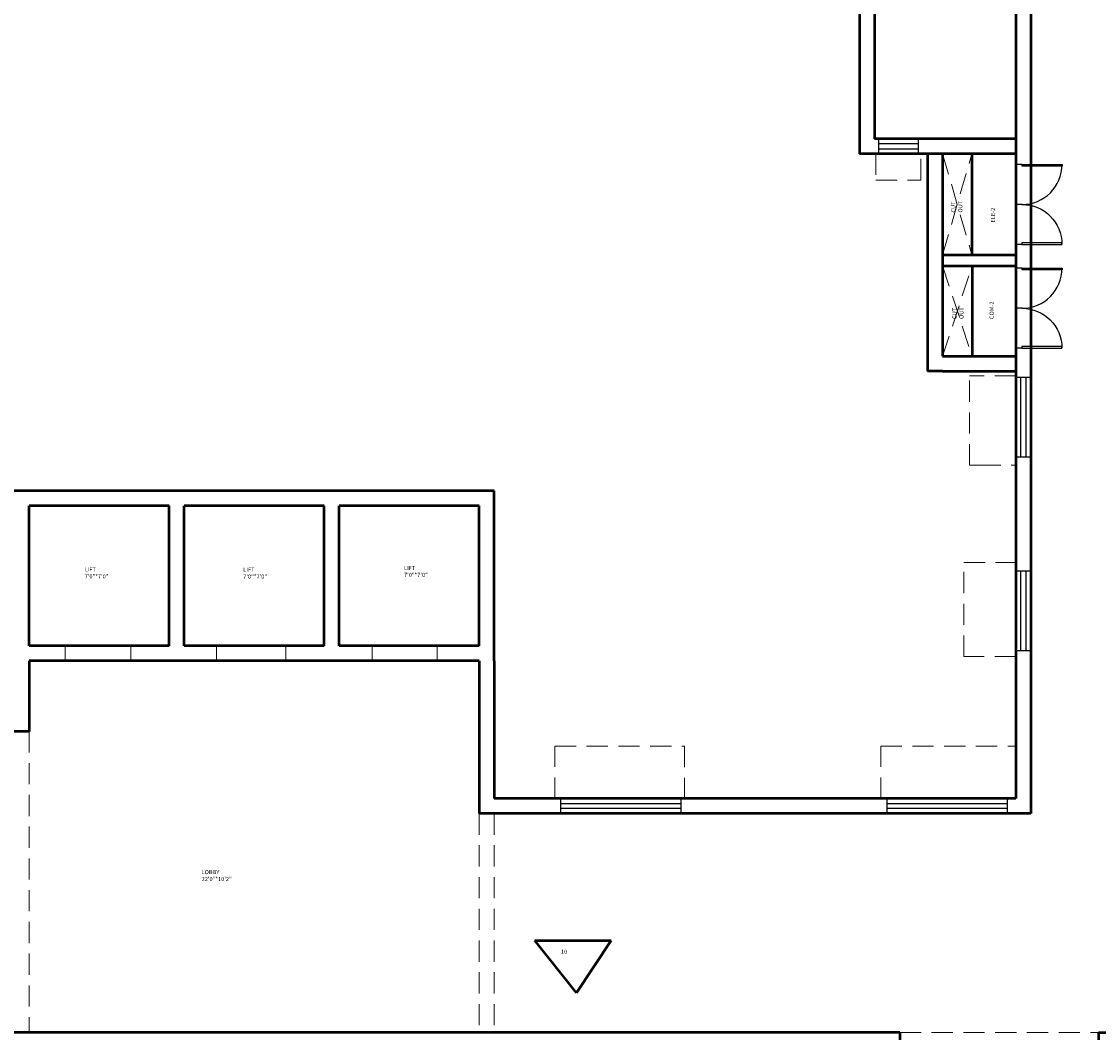
# Model space of a CAD drawing. Units: inches. Extents: x 291 to 2631, y 456 to 2623.
# Tile 9 of 22: x 1463 to 2109, y 931 to 1538. Entities that reach past the tile are written whole.
import ezdxf

# ---------------------------------------------------------------- set-up
doc = ezdxf.new("R2010")
doc.units = ezdxf.units.IN
doc.linetypes.add('DASHED', pattern=[19.05, 12.7, -6.35])
for name, color, linetype, lineweight in [('A-ANNO-TEXT', 3, 'Continuous', 25), ('A-AREA-IDEN', 7, 'Continuous', 25), ('A-DOOR', 3, 'Continuous', 25), ('A-FLOR-OVHD', 1, 'DASHED', 18), ('A-GLAZ', 4, 'Continuous', 25), ('A-WALL', 7, 'Continuous', 50)]:
    doc.layers.add(name, color=color, linetype=linetype, lineweight=lineweight)
doc.styles.get("Standard").update_dxf_attribs({"font": 'arial.ttf'})

# ---------------------------------------------------------------- blocks, each defined once
blk = doc.blocks.new('*U2')
for p, q in [((0, 0), (0, -6)), ((40, 0), (40, -6))]:
    blk.add_line(p, q)
blk.add_lwpolyline([(0, 0), (0, 40), (1.75, 40), (1.75, 0)], close=True)
blk.add_arc((0, 0), 40, 0, 90)
blk = doc.blocks.new('WIN-1800')
for p, q in [((0, 9), (72, 9)), ((0, 0), (0, 9)), ((72, 9), (72, 0)), ((0, 6), (72, 6)), ((72, 3), (0, 3)), ((72, 0), (0, 0))]:
    blk.add_line(p, q)
blk = doc.blocks.new('WIN-1200')
for p, q in [((0, 0), (0, 48)), ((0, 48), (9, 48)), ((3, 0), (3, 48)), ((6, 48), (6, 0)), ((9, 48), (9, 0)), ((9, 0), (0, 0))]:
    blk.add_line(p, q)
blk = doc.blocks.new('WIN-600')
for p, q in [((24, 9), (0, 9)), ((0, 9), (0, 0)), ((24, 0), (24, 9)), ((24, 6), (0, 6)), ((0, 3), (24, 3)), ((0, 0), (24, 0))]:
    blk.add_line(p, q)

msp = doc.modelspace()

# ---------------------------------------------------------------- linework, layer by layer
at = {"layer": 'A-FLOR-OVHD'}
for p, q in [((1975.46, 1458.32), (1975.46, 1442.5)), ((2002.48, 1442.5), (2002.48, 1458.32)), ((2015.46, 1458.32), (2033.04, 1397.55)), ((2015.46, 1397.55), (2033.04, 1458.32)), ((1975.46, 1442.5), (2002.48, 1442.5)), ((2015.46, 1390.95), (2033.18, 1336.78)), ((2015.46, 1336.78), (2033.18, 1390.95)), ((2031.54, 1271.35), (2031.54, 1325.01)), ((2031.54, 1325.01), (2037.66, 1325.01)), ((2059.49, 1325.01), (2037.66, 1325.01)), ((2037.66, 1271.35), (2031.54, 1271.35)), ((2037.66, 1271.35), (2059.49, 1271.35)), ((2028.23, 1156.55), (2028.23, 1213.02)), ((2028.23, 1213.02), (2059.49, 1213.02)), ((1489.28, 1163.05), (1489.28, 1154.05)), ((1528.71, 1163.05), (1528.71, 1154.05)), ((1580.01, 1163.05), (1580.01, 1154.05)), ((1621.53, 1163.05), (1621.53, 1154.05)), ((1673.4, 1163.05), (1673.4, 1154.05)), ((1712.4, 1163.05), (1712.4, 1154.05)), ((2059.49, 1156.55), (2028.23, 1156.55)), ((1467.6, 1111.65), (1467.6, 930.98)), ((1782.97, 1071.35), (1782.97, 1102.83)), ((1782.97, 1102.83), (1860.62, 1102.83)), ((1860.62, 1102.83), (1860.62, 1071.35)), ((1978.37, 1071.35), (1978.37, 1102.83)), ((1978.37, 1102.83), (2059.49, 1102.83)), ((1737.6, 1062.35), (1737.6, 930.98)), ((1746.6, 1062.35), (1746.6, 930.98)), ((1989.87, 930.98), (2108.97, 930.98))]:
    msp.add_line(p, q, dxfattribs=at)
at = {"layer": 'A-WALL'}
for p, q in [((1965.72, 1754.24), (1965.72, 1458.32)), ((1974.72, 1754.24), (1974.72, 1467.32)), ((2059.49, 1754.24), (2059.49, 1490.6)), ((2068.49, 1754.24), (2068.49, 1489.98)), ((2059.49, 1490.6), (2059.49, 1071.35)), ((2068.49, 1489.98), (2068.49, 1062.35)), ((2059.49, 1467.32), (1974.72, 1467.32)), ((2059.49, 1458.32), (1965.72, 1458.32)), ((2006.46, 1458.32), (2006.46, 1327.78)), ((2015.46, 1458.32), (2015.46, 1336.78)), ((2033.04, 1458.32), (2033.04, 1397.55)), ((2015.46, 1397.55), (2059.49, 1397.55)), ((2015.46, 1390.95), (2059.49, 1390.95)), ((2033.18, 1390.95), (2033.18, 1336.78)), ((2015.46, 1336.78), (2059.49, 1336.78)), ((2015.46, 1327.78), (2006.46, 1327.78)), ((2015.46, 1327.78), (2059.49, 1327.78)), ((1746.6, 1256.05), (1120.83, 1256.05)), ((1746.6, 1220), (1746.6, 1256.05)), ((1467.6, 1220), (1467.6, 1247.05)), ((1551.6, 1247.05), (1467.6, 1247.05)), ((1551.6, 1220), (1551.6, 1247.05)), ((1560.6, 1220), (1560.6, 1247.05)), ((1644.6, 1247.05), (1560.6, 1247.05)), ((1644.6, 1220), (1644.6, 1247.05)), ((1737.6, 1247.05), (1653.6, 1247.05)), ((1653.6, 1220), (1653.6, 1247.05)), ((1737.6, 1220), (1737.6, 1247.05)), ((1467.6, 1163.05), (1467.6, 1220)), ((1551.6, 1163.05), (1551.6, 1220)), ((1560.6, 1163.05), (1560.6, 1220)), ((1644.6, 1163.05), (1644.6, 1220)), ((1653.6, 1163.05), (1653.6, 1220)), ((1737.6, 1163.05), (1737.6, 1220)), ((1746.6, 1154.05), (1746.6, 1220)), ((1551.6, 1163.05), (1467.6, 1163.05)), ((1644.6, 1163.05), (1560.6, 1163.05)), ((1737.6, 1163.05), (1653.6, 1163.05)), ((1737.6, 1154.05), (1467.6, 1154.05)), ((1467.6, 1154.05), (1467.6, 1111.65)), ((1737.6, 1154.05), (1737.6, 1062.35)), ((1746.6, 1154.05), (1746.6, 1071.35)), ((1467.6, 1111.65), (1032.82, 1111.65)), ((2059.49, 1071.35), (1746.6, 1071.35)), ((2068.49, 1062.35), (1737.6, 1062.35)), ((1770.87, 986.26), (1816.68, 986.26)), ((1796, 954.68), (1770.87, 986.26)), ((1816.68, 986.26), (1796, 954.68)), ((1989.87, 930.98), (1024, 930.98)), ((1989.87, 930.98), (1989.87, 801.98)), ((2108.97, 930.98), (2168.21, 930.98)), ((2108.97, 930.98), (2108.97, 527.48))]:
    msp.add_line(p, q, dxfattribs=at)

# ---------------------------------------------------------------- block references
at = {"layer": 'A-DOOR', "yscale": 0.6, "zscale": 0.6, "rotation": 270}
for p, xscale in [((2063.14, 1451.85), 0.6), ((2063.09, 1403.85), -0.6), ((2063.14, 1389.59), 0.6), ((2063.09, 1341.59), -0.6)]:
    msp.add_blockref('*U2', p, dxfattribs=dict(at, xscale=xscale))
at = {"layer": 'A-GLAZ', "rotation": 180}
for name, p in [('WIN-600', (2000.98, 1467.32)), ('WIN-1200', (2068.49, 1324.16)), ('WIN-1200', (2068.49, 1208.08))]:
    msp.add_blockref(name, p, dxfattribs=at)
at = {"layer": 'A-GLAZ'}
for p in [(1786.47, 1062.35), (1982.3, 1062.35)]:
    msp.add_blockref('WIN-1800', p, dxfattribs=at)

# ---------------------------------------------------------------- texts
at = {"layer": 'A-ANNO-TEXT', "char_height": 2.5, "attachment_point": 1, "rotation": 90}
for s, width, insert in [('CUT OUT', 12.6397, (2020.72, 1423)), ('COM-2', 18.6435, (2043.69, 1359.07)), ('CUT\\POUT', 13.1406, (2021.37, 1359.15))]:
    msp.add_mtext_dynamic_manual_height_columns(s, width=width, gutter_width=12.5, heights=[0], dxfattribs=dict(at, insert=insert))
at = {"layer": 'A-ANNO-TEXT', "insert": (1786.61, 980.68), "char_height": 2.5, "attachment_point": 1}
msp.add_mtext_dynamic_manual_height_columns('10', width=13.8695, gutter_width=12.5, heights=[0], dxfattribs=at)
at = {"layer": 'A-AREA-IDEN', "insert": (2044.43, 1417.01), "char_height": 2.5, "attachment_point": 1, "rotation": 90}
msp.add_mtext_dynamic_manual_height_columns('ELE-2', width=19.0468, gutter_width=12.5, heights=[0], dxfattribs=at)
at = {"layer": 'A-AREA-IDEN', "char_height": 2.5, "attachment_point": 1}
for s, width, insert in [('LIFT\\P7\'0"*7\'0"', 43.7041, (1500.94, 1210.13)), ('LIFT\\P7\'0"*7\'0"', 43.7041, (1596.05, 1209.97)), ('LIFT\\P7\'0"*7\'0"', 43.7041, (1692.47, 1210.98)), ('LOBBY\\P22\'0"*10\'2"', 179.3086, (1571.09, 1028.48))]:
    msp.add_mtext_dynamic_manual_height_columns(s, width=width, gutter_width=12.5, heights=[0], dxfattribs=dict(at, insert=insert))

doc.saveas('drawing.dxf')
